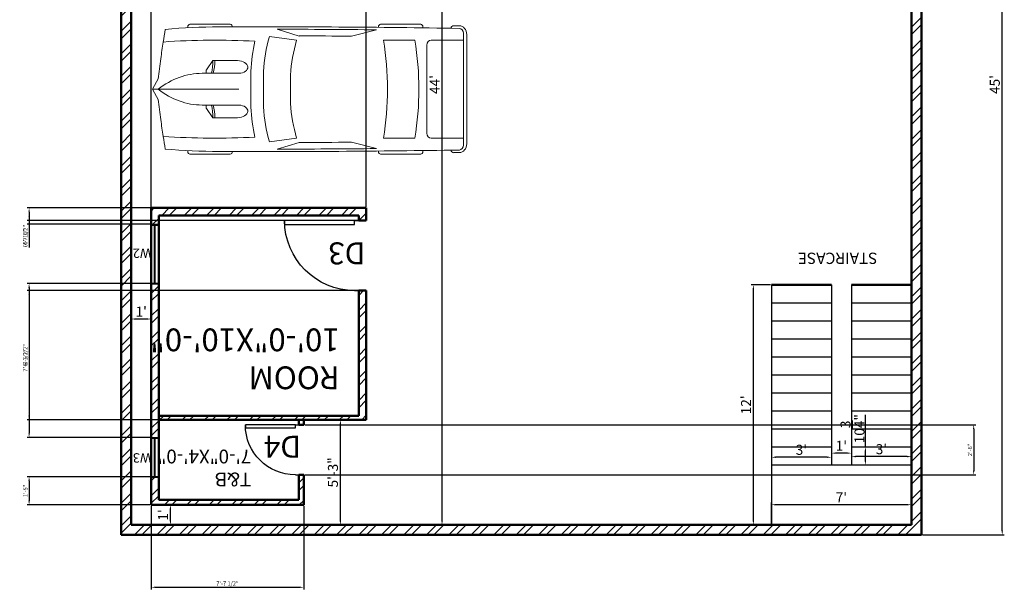
# Model space of a CAD drawing. Units: inches. Extents: x 244 to 2800, y 1060 to 1700.
# Tile 12 of 13: x 2210 to 2800, y 1060 to 1402. Entities that reach past the tile are written whole.
import ezdxf

# ---------------------------------------------------------------- set-up
doc = ezdxf.new("R2010")
doc.units = ezdxf.units.IN
for name, color, linetype, lineweight in [('A-ANNO-DIMS', 2, 'Continuous', 18), ('A-ANNO-TEXT', 1, 'Continuous', 18), ('A-DOOR', 5, 'Continuous', 25), ('A-FLOR-STRS', 6, 'Continuous', 25), ('A-FURN', 9, 'Continuous', 18), ('A-GLAZ', 3, 'Continuous', 25), ('A-WALL', 7, 'Continuous', 50), ('A-WALL-PATT', 8, 'Continuous', 13)]:
    doc.layers.add(name, color=color, linetype=linetype, lineweight=lineweight)
doc.styles.get("Standard").update_dxf_attribs({"font": 'arial.ttf'})
doc.dimstyles.new('ISO-25', dxfattribs={"dimtxt": 2.5, "dimasz": 2.5, "dimexe": 1.25, "dimexo": 0.625, "dimtad": 1, "dimlunit": 4, "dimtxsty": 'Standard', "dimcen": 2.5, "dimadec": 0, "dimazin": 0, "dimtfac": 1, "dimtmove": 0, "dimatfit": 3, "dimfxl": 1, "dimarcsym": 0})

# ---------------------------------------------------------------- blocks, each defined once
blk = doc.blocks.new('*U2')
for p, q in [((0, 0), (0, -5)), ((30, 0), (30, -5))]:
    blk.add_line(p, q)
blk.add_lwpolyline([(0, 0), (0, 30), (1.75, 30), (1.75, 0)], close=True)
blk.add_arc((0, 0), 30, 0, 90)
blk = doc.blocks.new('*D9')
at = {"layer": 'A-ANNO-DIMS', "color": 0, "lineweight": -2, "transparency": 16777216}
for p, q in [((2751.08, 1632.99), (2800.17, 1632.99)), ((2798.92, 1095.49), (2798.92, 1630.49)), ((2751.08, 1092.99), (2800.17, 1092.99))]:
    blk.add_line(p, q, dxfattribs=at)
at = {"layer": 'A-ANNO-DIMS', "color": 0, "transparency": 16777216}
for points in [[(2798.5, 1630.49), (2799.34, 1630.49), (2798.92, 1632.99)], [(2798.5, 1095.49), (2799.34, 1095.49), (2798.92, 1092.99)]]:
    blk.add_solid(points, dxfattribs=at)
at = {"layer": 'Defpoints', "color": 0, "transparency": 16777216}
for p in [(2750.46, 1632.99), (2798.92, 1632.99), (2750.46, 1092.99)]:
    blk.add_point(p, dxfattribs=at)
at = {"layer": 'A-ANNO-DIMS', "color": 0, "transparency": 16777216, "insert": (2795.24, 1362.99), "char_height": 6, "attachment_point": 5, "rotation": 90}
blk.add_mtext("45'", dxfattribs=at)
blk = doc.blocks.new('*D15')
at = {"layer": 'A-ANNO-DIMS', "color": 0, "lineweight": -2, "transparency": 16777216}
for p, q in [((2276.46, 1216.94), (2276.46, 1223.68)), ((2288.46, 1216.94), (2288.46, 1223.68)), ((2285.96, 1222.43), (2278.96, 1222.43))]:
    blk.add_line(p, q, dxfattribs=at)
at = {"layer": 'A-ANNO-DIMS', "color": 0, "transparency": 16777216}
for points in [[(2278.96, 1222.84), (2278.96, 1222.01), (2276.46, 1222.43)], [(2285.96, 1222.84), (2285.96, 1222.01), (2288.46, 1222.43)]]:
    blk.add_solid(points, dxfattribs=at)
at = {"layer": 'Defpoints', "color": 0, "transparency": 16777216}
for p in [(2276.46, 1222.43), (2276.46, 1216.32), (2288.46, 1216.32)]:
    blk.add_point(p, dxfattribs=at)
at = {"layer": 'A-ANNO-DIMS', "color": 0, "transparency": 16777216, "insert": (2282.46, 1226.06), "char_height": 6, "attachment_point": 5}
blk.add_mtext("1'", dxfattribs=at)
blk = doc.blocks.new('*D16')
at = {"layer": 'A-ANNO-DIMS', "color": 0, "lineweight": -2, "transparency": 16777216}
for p, q in [((2305.77, 1110.99), (2298.74, 1110.99)), ((2299.99, 1101.49), (2299.99, 1108.49)), ((2305.77, 1098.99), (2298.74, 1098.99))]:
    blk.add_line(p, q, dxfattribs=at)
at = {"layer": 'A-ANNO-DIMS', "color": 0, "transparency": 16777216}
for points in [[(2299.57, 1108.49), (2300.41, 1108.49), (2299.99, 1110.99)], [(2299.57, 1101.49), (2300.41, 1101.49), (2299.99, 1098.99)]]:
    blk.add_solid(points, dxfattribs=at)
at = {"layer": 'Defpoints', "color": 0, "transparency": 16777216}
for p in [(2299.99, 1110.99), (2306.39, 1110.99), (2306.39, 1098.99)]:
    blk.add_point(p, dxfattribs=at)
at = {"layer": 'A-ANNO-DIMS', "color": 0, "transparency": 16777216, "insert": (2296.35, 1104.99), "char_height": 6, "attachment_point": 5, "rotation": 90}
blk.add_mtext("1'", dxfattribs=at)
blk = doc.blocks.new('*D18')
at = {"layer": 'A-ANNO-DIMS', "color": 0, "lineweight": -2, "transparency": 16777216}
for p, q in [((2660.46, 1099.61), (2660.46, 1112.37)), ((2741.96, 1111.12), (2662.96, 1111.12)), ((2744.46, 1099.61), (2744.46, 1112.37))]:
    blk.add_line(p, q, dxfattribs=at)
at = {"layer": 'A-ANNO-DIMS', "color": 0, "transparency": 16777216}
for points in [[(2662.96, 1111.54), (2662.96, 1110.7), (2660.46, 1111.12)], [(2741.96, 1111.54), (2741.96, 1110.7), (2744.46, 1111.12)]]:
    blk.add_solid(points, dxfattribs=at)
at = {"layer": 'Defpoints', "color": 0, "transparency": 16777216}
for p in [(2660.46, 1111.12), (2660.46, 1098.99), (2744.46, 1098.99)]:
    blk.add_point(p, dxfattribs=at)
at = {"layer": 'A-ANNO-DIMS', "color": 0, "transparency": 16777216, "insert": (2702.46, 1114.74), "char_height": 6, "attachment_point": 5}
blk.add_mtext("7'", dxfattribs=at)
blk = doc.blocks.new('*D19')
at = {"layer": 'A-ANNO-DIMS', "color": 0, "lineweight": -2, "transparency": 16777216}
for p, q in [((2708.46, 1145.16), (2708.46, 1138.69)), ((2741.96, 1139.94), (2710.96, 1139.94)), ((2744.46, 1145.16), (2744.46, 1138.69))]:
    blk.add_line(p, q, dxfattribs=at)
at = {"layer": 'A-ANNO-DIMS', "color": 0, "transparency": 16777216}
for points in [[(2710.96, 1140.36), (2710.96, 1139.52), (2708.46, 1139.94)], [(2741.96, 1140.36), (2741.96, 1139.52), (2744.46, 1139.94)]]:
    blk.add_solid(points, dxfattribs=at)
at = {"layer": 'Defpoints', "color": 0, "transparency": 16777216}
for p in [(2708.46, 1145.79), (2744.46, 1145.79), (2708.46, 1139.94)]:
    blk.add_point(p, dxfattribs=at)
at = {"layer": 'A-ANNO-DIMS', "color": 0, "transparency": 16777216, "insert": (2726.46, 1143.63), "char_height": 6, "attachment_point": 5}
blk.add_mtext("3'", dxfattribs=at)
blk = doc.blocks.new('*D20')
at = {"layer": 'A-ANNO-DIMS', "color": 0, "lineweight": -2, "transparency": 16777216}
for p, q in [((2716.85, 1145.79), (2716.85, 1165.08)), ((2709.08, 1145.79), (2718.1, 1145.79)), ((2716.85, 1137.49), (2716.85, 1143.29)), ((2709.08, 1134.99), (2718.1, 1134.99))]:
    blk.add_line(p, q, dxfattribs=at)
at = {"layer": 'A-ANNO-DIMS', "color": 0, "transparency": 16777216}
for points in [[(2716.43, 1143.29), (2717.27, 1143.29), (2716.85, 1145.79)], [(2716.43, 1137.49), (2717.27, 1137.49), (2716.85, 1134.99)]]:
    blk.add_solid(points, dxfattribs=at)
at = {"layer": 'Defpoints', "color": 0, "transparency": 16777216}
for p in [(2708.46, 1145.79), (2716.85, 1145.79), (2708.46, 1134.99)]:
    blk.add_point(p, dxfattribs=at)
at = {"layer": 'A-ANNO-DIMS', "color": 0, "transparency": 16777216, "insert": (2709.11, 1156.68), "char_height": 6, "attachment_point": 5, "rotation": 90}
blk.add_mtext('10{\\H1x;\\S3/4;}"', dxfattribs=at)
blk = doc.blocks.new('*D21')
at = {"layer": 'A-ANNO-DIMS', "color": 0, "lineweight": -2, "transparency": 16777216}
for p, q in [((2696.46, 1145.16), (2696.46, 1140.78)), ((2705.96, 1142.03), (2698.96, 1142.03)), ((2708.46, 1145.16), (2708.46, 1140.78))]:
    blk.add_line(p, q, dxfattribs=at)
at = {"layer": 'A-ANNO-DIMS', "color": 0, "transparency": 16777216}
for points in [[(2698.96, 1142.45), (2698.96, 1141.62), (2696.46, 1142.03)], [(2705.96, 1142.45), (2705.96, 1141.62), (2708.46, 1142.03)]]:
    blk.add_solid(points, dxfattribs=at)
at = {"layer": 'Defpoints', "color": 0, "transparency": 16777216}
for p in [(2696.46, 1145.79), (2708.46, 1145.79), (2696.46, 1142.03)]:
    blk.add_point(p, dxfattribs=at)
at = {"layer": 'A-ANNO-DIMS', "color": 0, "transparency": 16777216, "insert": (2702.46, 1145.67), "char_height": 6, "attachment_point": 5}
blk.add_mtext("1'", dxfattribs=at)
blk = doc.blocks.new('*D22')
at = {"layer": 'A-ANNO-DIMS', "color": 0, "lineweight": -2, "transparency": 16777216}
for p, q in [((2660.46, 1143.51), (2660.46, 1138.32)), ((2696.46, 1143.51), (2696.46, 1138.32)), ((2693.96, 1139.57), (2662.96, 1139.57))]:
    blk.add_line(p, q, dxfattribs=at)
at = {"layer": 'A-ANNO-DIMS', "color": 0, "transparency": 16777216}
for points in [[(2662.96, 1139.99), (2662.96, 1139.16), (2660.46, 1139.57)], [(2693.96, 1139.99), (2693.96, 1139.16), (2696.46, 1139.57)]]:
    blk.add_solid(points, dxfattribs=at)
at = {"layer": 'Defpoints', "color": 0, "transparency": 16777216}
for p in [(2660.46, 1144.13), (2696.46, 1144.13), (2660.46, 1139.57)]:
    blk.add_point(p, dxfattribs=at)
at = {"layer": 'A-ANNO-DIMS', "color": 0, "transparency": 16777216, "insert": (2678.46, 1143.26), "char_height": 6, "attachment_point": 5}
blk.add_mtext("3'", dxfattribs=at)
blk = doc.blocks.new('*D23')
at = {"layer": 'A-ANNO-DIMS', "color": 0, "lineweight": -2, "transparency": 16777216}
for p, q in [((2659.83, 1242.99), (2648.4, 1242.99)), ((2649.65, 1101.49), (2649.65, 1240.49)), ((2659.83, 1098.99), (2648.4, 1098.99))]:
    blk.add_line(p, q, dxfattribs=at)
at = {"layer": 'A-ANNO-DIMS', "color": 0, "transparency": 16777216}
for points in [[(2649.24, 1240.49), (2650.07, 1240.49), (2649.65, 1242.99)], [(2649.24, 1101.49), (2650.07, 1101.49), (2649.65, 1098.99)]]:
    blk.add_solid(points, dxfattribs=at)
at = {"layer": 'Defpoints', "color": 0, "transparency": 16777216}
for p in [(2649.65, 1242.99), (2660.46, 1242.99), (2660.46, 1098.99)]:
    blk.add_point(p, dxfattribs=at)
at = {"layer": 'A-ANNO-DIMS', "color": 0, "transparency": 16777216, "insert": (2646.02, 1170.99), "char_height": 6, "attachment_point": 5, "rotation": 90}
blk.add_mtext("12'", dxfattribs=at)
blk = doc.blocks.new('*D24')
at = {"layer": 'A-ANNO-DIMS', "color": 0, "lineweight": -2, "transparency": 16777216}
for p, q in [((2407.43, 1161.99), (2400.69, 1161.99)), ((2401.94, 1101.49), (2401.94, 1159.49)), ((2407.43, 1098.99), (2400.69, 1098.99))]:
    blk.add_line(p, q, dxfattribs=at)
at = {"layer": 'A-ANNO-DIMS', "color": 0, "transparency": 16777216}
for points in [[(2401.52, 1159.49), (2402.36, 1159.49), (2401.94, 1161.99)], [(2401.52, 1101.49), (2402.36, 1101.49), (2401.94, 1098.99)]]:
    blk.add_solid(points, dxfattribs=at)
at = {"layer": 'Defpoints', "color": 0, "transparency": 16777216}
for p in [(2401.94, 1161.99), (2408.06, 1161.99), (2408.06, 1098.99)]:
    blk.add_point(p, dxfattribs=at)
at = {"layer": 'A-ANNO-DIMS', "color": 0, "transparency": 16777216, "insert": (2398.25, 1130.49), "char_height": 6, "attachment_point": 5, "rotation": 90}
blk.add_mtext('5\'-3"', dxfattribs=at)
blk = doc.blocks.new('*D45')
at = {"layer": 'A-ANNO-DIMS', "color": 0, "lineweight": -2, "transparency": 16777216}
for p, q in [((2478.2, 1626.99), (2461.68, 1626.99)), ((2462.93, 1101.49), (2462.93, 1624.49)), ((2478.2, 1098.99), (2461.68, 1098.99))]:
    blk.add_line(p, q, dxfattribs=at)
at = {"layer": 'A-ANNO-DIMS', "color": 0, "transparency": 16777216}
for points in [[(2462.51, 1624.49), (2463.34, 1624.49), (2462.93, 1626.99)], [(2462.51, 1101.49), (2463.34, 1101.49), (2462.93, 1098.99)]]:
    blk.add_solid(points, dxfattribs=at)
at = {"layer": 'Defpoints', "color": 0, "transparency": 16777216}
for p in [(2462.93, 1626.99), (2478.82, 1626.99), (2478.82, 1098.99)]:
    blk.add_point(p, dxfattribs=at)
at = {"layer": 'A-ANNO-DIMS', "color": 0, "transparency": 16777216, "insert": (2459.3, 1362.99), "char_height": 6, "attachment_point": 5, "rotation": 90}
blk.add_mtext("44'", dxfattribs=at)
blk = doc.blocks.new('*U47')
for p, q in [((21.1, 37.41), (21.1, 36.83)), ((46.55, 38.89), (22.35, 38.89)), ((47.8, 37.39), (47.8, 37.41)), ((87.99, 31.87), (74.76, 35.92)), ((134.31, 35.6), (119.29, 31.78)), ((135.45, 37.07), (135.45, 37.41)), ((136.7, 38.89), (160.9, 38.89)), ((162.15, 37.41), (162.15, 36.77)), ((70.03, 31.54), (86.41, 29.35)), ((186.47, -33.5), (186.47, 33.5)), ((188.4, -32.76), (188.4, 32.76)), ((138.42, 29.35), (157.25, 29.35)), ((164.52, 26.39), (164.52, -26.39)), ((186.47, 29.35), (167.01, 29.35)), ((32.27, 11.63), (36.13, 17.17)), ((36.13, 17.17), (50.94, 17.17)), ((3.27, 6.13), (0.1, 0.41)), ((29.77, 9.51), (51.68, 9.51)), ((32.12, 9.51), (32.12, 11.15)), ((58.92, -10.77), (58.92, 10.77)), ((66.55, -10.53), (66.55, 10.53)), ((82.74, 8.5), (82.74, -8.5)), ((186.47, -10.53), (186.47, 10.53)), ((0, 0), (51.68, 0)), ((0.1, -0.41), (3.27, -6.13)), ((29.77, -9.51), (51.68, -9.51)), ((32.12, -9.51), (32.12, -11.15)), ((32.27, -11.63), (36.13, -17.17)), ((36.13, -17.17), (50.94, -17.17)), ((86.41, -29.35), (70.03, -31.54)), ((157.25, -29.35), (138.42, -29.35)), ((167.01, -29.35), (186.47, -29.35)), ((87.99, -31.87), (74.76, -35.92)), ((134.31, -35.6), (119.29, -31.78)), ((21.1, -37.41), (21.1, -36.83)), ((46.55, -38.89), (22.35, -38.89)), ((47.8, -37.39), (47.8, -37.41)), ((135.45, -37.07), (135.45, -37.41)), ((136.7, -38.89), (160.9, -38.89)), ((162.15, -37.41), (162.15, -36.77))]:
    blk.add_line(p, q)
for centre, major_axis, ratio, start_param, end_param in [((266.03, -27.52), (0, 313.31), 0.842304, 1.367076, 1.39176), ((41.19, -490.86), (0, 528.23), 0.842304, 0.00281, 0.075598), ((22.35, 37.41), (0, -1.48), 0.842304, 3.141593, 4.712389), ((64.48, -10555.62), (0, 10593.03), 0.842304, -0.013397, 0.002797), ((46.55, 37.41), (0, 1.48), 0.842304, -1.570796, 0), ((64.48, -10555.62), (0, -10591.55), 0.842304, 3.133765, 3.140441), ((136.7, 37.41), (0, -1.48), 0.842304, 3.141593, 4.712389), ((160.9, 37.41), (0, 1.48), 0.842304, -1.570796, 0), ((180.63, 35.84), (0, 2.22), 0.842304, -0.013017, 1.249894), ((64.48, -10556.36), (0, 10595.31), 0.842304, -0.013397, -0.013017), ((183.98, 33.5), (0, -2.96), 0.842304, 1.570796, 3.128196), ((183.98, 32.76), (0, -5.25), 0.842304, 1.570796, 3.128196), ((37.47, -593.96), (0, -623.33), 0.842304, 3.096046, 3.200911), ((135.29, 5.39), (0, 81.77), 0.842304, 1.245306, 1.50788), ((95.79, -3666.35), (0, -3698.24), 0.842304, 3.134049, 3.144098), ((259.18, -27.52), (0, -305.3), 0.842304, 4.528606, 4.561838), ((134.4, 5.39), (0, -89.78), 0.842304, 4.449482, 4.652344), ((149.6, 2.8), (0, -79.58), 0.842304, 4.372215, 4.640744), ((17.08, 0), (0, 147.02), 0.842304, 4.511394, 4.913384), ((35.91, 0), (0, 147.02), 0.842304, 4.511394, 4.913384), ((167.01, 26.39), (0, 2.96), 0.842304, 0, 1.570796), ((-204.49, 52.4), (0, -250.96), 0.842304, 1.385369, 1.434372), ((13.04, 17.01), (0, 27.42), 0.842304, 4.435146, 4.718221), ((14.2, 17.01), (0, 27.42), 0.842304, 4.435146, 4.718221), ((50.79, 13.34), (6.34, -0.36), 0.603834, -1.395552, 1.581315), ((29.77, -46.66), (0, 56.17), 0.842304, 0, 0.590319), ((32.75, 11.15), (0, 0.74), 0.842304, 0.879714, 1.570796), ((0.62, 0), (0, -0.74), 0.842304, 4.131459, 5.293319), ((29.77, 46.66), (0, 56.17), 0.842304, 2.551274, 3.141593), ((-204.49, -52.4), (0, 250.96), 0.842304, -1.434372, -1.385369), ((32.75, -11.15), (0, -0.74), 0.842304, 4.712389, 5.403472), ((13.04, -17.01), (0, -27.42), 0.842304, 1.564964, 1.848039), ((14.2, -17.01), (0, -27.42), 0.842304, 1.564964, 1.848039), ((134.4, -5.39), (0, -89.78), 0.842304, -1.510751, -1.307889), ((135.29, -5.39), (0, -81.77), 0.842304, -1.50788, -1.245306), ((149.6, -2.8), (0, -79.58), 0.842304, -1.499151, -1.230623), ((259.18, 27.52), (0, 305.3), 0.842304, 1.721348, 1.754579), ((266.03, 27.52), (0, 313.31), 0.842304, 1.749832, 1.774517), ((37.47, 593.96), (0, -623.33), 0.842304, -0.059319, 0.045547), ((167.01, -26.39), (0, -2.96), 0.842304, 4.712389, 6.283185), ((95.79, 3666.35), (0, -3698.24), 0.842304, -0.002505, 0.007544), ((183.98, -33.5), (0, 2.96), 0.842304, 3.15499, 4.712389), ((183.98, -32.76), (0, -5.25), 0.842304, 0.013397, 1.570796), ((41.19, 490.86), (0, -528.23), 0.842304, -0.075598, -0.00281), ((22.35, -37.41), (0, 1.48), 0.842304, 1.570796, 3.141593), ((64.48, 10555.62), (0, 10593.03), 0.842304, 3.138796, 3.15499), ((46.55, -37.41), (0, -1.48), 0.842304, 0, 1.570796), ((64.48, 10555.62), (0, -10591.55), 0.842304, 0.001152, 0.007828), ((136.7, -37.41), (0, -1.48), 0.842304, -1.570796, 0), ((160.9, -37.41), (0, 1.48), 0.842304, 3.141593, 4.712389), ((180.63, -35.84), (0, -2.22), 0.842304, -1.249894, 0.013017), ((64.48, 10556.36), (0, 10595.31), 0.842304, 3.15461, 3.15499)]:
    blk.add_ellipse(centre, major_axis=major_axis, ratio=ratio, start_param=start_param, end_param=end_param)
at = {"extrusion": (0, 0, -1)}
blk.add_ellipse((50.79, -13.34), major_axis=(6.34, 0.36), ratio=0.603834, start_param=-1.395552, end_param=1.581315, dxfattribs=at)
blk = doc.blocks.new('*D148')
at = {"layer": 'A-ANNO-DIMS', "color": 0, "lineweight": -2, "transparency": 16777216}
for p, q in [((2288.46, 1289.61), (2288.46, 1665.59)), ((2417.46, 1289.61), (2417.46, 1665.59)), ((2290.96, 1664.34), (2414.96, 1664.34))]:
    blk.add_line(p, q, dxfattribs=at)
at = {"layer": 'A-ANNO-DIMS', "color": 0, "transparency": 16777216}
for points in [[(2290.96, 1664.75), (2290.96, 1663.92), (2288.46, 1664.34)], [(2414.96, 1664.75), (2414.96, 1663.92), (2417.46, 1664.34)]]:
    blk.add_solid(points, dxfattribs=at)
at = {"layer": 'Defpoints', "color": 0, "transparency": 16777216}
for p in [(2417.46, 1664.34), (2288.46, 1288.99), (2417.46, 1288.99)]:
    blk.add_point(p, dxfattribs=at)
at = {"layer": 'A-ANNO-DIMS', "color": 0, "transparency": 16777216, "insert": (2352.96, 1666.24), "char_height": 2.5, "attachment_point": 5}
blk.add_mtext('10\'-9"', dxfattribs=at)
blk = doc.blocks.new('*D149')
at = {"layer": 'A-ANNO-DIMS', "color": 0, "lineweight": -2, "transparency": 16777216}
for p, q in [((2287.83, 1288.99), (2213.97, 1288.99)), ((2215.22, 1286.49), (2215.22, 1281.7)), ((2287.83, 1279.2), (2213.97, 1279.2)), ((2215.22, 1279.2), (2215.22, 1266.86))]:
    blk.add_line(p, q, dxfattribs=at)
at = {"layer": 'A-ANNO-DIMS', "color": 0, "transparency": 16777216}
for points in [[(2214.81, 1286.49), (2215.64, 1286.49), (2215.22, 1288.99)], [(2214.81, 1281.7), (2215.64, 1281.7), (2215.22, 1279.2)]]:
    blk.add_solid(points, dxfattribs=at)
at = {"layer": 'Defpoints', "color": 0, "transparency": 16777216}
for p in [(2288.46, 1288.99), (2215.22, 1279.2), (2288.46, 1279.2)]:
    blk.add_point(p, dxfattribs=at)
at = {"layer": 'A-ANNO-DIMS', "color": 0, "transparency": 16777216, "insert": (2213.32, 1271.78), "char_height": 2.5, "attachment_point": 5, "rotation": 90}
blk.add_mtext('0\'-10"', dxfattribs=at)
blk = doc.blocks.new('*D150')
at = {"layer": 'A-ANNO-DIMS', "color": 0, "lineweight": -2, "transparency": 16777216}
for p, q in [((2287.83, 1243.73), (2213.97, 1243.73)), ((2215.22, 1241.23), (2215.22, 1153.92)), ((2287.83, 1151.42), (2213.97, 1151.42))]:
    blk.add_line(p, q, dxfattribs=at)
at = {"layer": 'A-ANNO-DIMS', "color": 0, "transparency": 16777216}
for points in [[(2214.81, 1241.23), (2215.64, 1241.23), (2215.22, 1243.73)], [(2214.81, 1153.92), (2215.64, 1153.92), (2215.22, 1151.42)]]:
    blk.add_solid(points, dxfattribs=at)
at = {"layer": 'Defpoints', "color": 0, "transparency": 16777216}
for p in [(2288.46, 1243.73), (2215.22, 1151.42), (2288.46, 1151.42)]:
    blk.add_point(p, dxfattribs=at)
at = {"layer": 'A-ANNO-DIMS', "color": 0, "transparency": 16777216, "insert": (2213.31, 1197.57), "char_height": 2.5, "attachment_point": 5, "rotation": 90}
blk.add_mtext('7\'-8 1/2"', dxfattribs=at)
blk = doc.blocks.new('*D151')
at = {"layer": 'A-ANNO-DIMS', "color": 0, "lineweight": -2, "transparency": 16777216}
for p, q in [((2287.83, 1127.9), (2213.97, 1127.9)), ((2215.22, 1125.4), (2215.22, 1113.49)), ((2287.83, 1110.99), (2213.97, 1110.99))]:
    blk.add_line(p, q, dxfattribs=at)
at = {"layer": 'A-ANNO-DIMS', "color": 0, "transparency": 16777216}
for points in [[(2214.81, 1125.4), (2215.64, 1125.4), (2215.22, 1127.9)], [(2214.81, 1113.49), (2215.64, 1113.49), (2215.22, 1110.99)]]:
    blk.add_solid(points, dxfattribs=at)
at = {"layer": 'Defpoints', "color": 0, "transparency": 16777216}
for p in [(2288.46, 1127.9), (2215.22, 1110.99), (2288.46, 1110.99)]:
    blk.add_point(p, dxfattribs=at)
at = {"layer": 'A-ANNO-DIMS', "color": 0, "transparency": 16777216, "insert": (2213.32, 1119.44), "char_height": 2.5, "attachment_point": 5, "rotation": 90}
blk.add_mtext('1\'-5"', dxfattribs=at)
blk = doc.blocks.new('*D152')
at = {"layer": 'A-ANNO-DIMS', "color": 0, "lineweight": -2, "transparency": 16777216}
for p, q in [((2416.83, 1288.99), (2213.97, 1288.99)), ((2215.22, 1286.49), (2215.22, 1283.99)), ((2416.83, 1281.49), (2213.97, 1281.49)), ((2215.22, 1281.49), (2215.22, 1265.27))]:
    blk.add_line(p, q, dxfattribs=at)
at = {"layer": 'A-ANNO-DIMS', "color": 0, "transparency": 16777216}
for points in [[(2214.81, 1286.49), (2215.64, 1286.49), (2215.22, 1288.99)], [(2214.81, 1283.99), (2215.64, 1283.99), (2215.22, 1281.49)]]:
    blk.add_solid(points, dxfattribs=at)
at = {"layer": 'Defpoints', "color": 0, "transparency": 16777216}
for p in [(2417.46, 1288.99), (2215.22, 1281.49), (2417.46, 1281.49)]:
    blk.add_point(p, dxfattribs=at)
at = {"layer": 'A-ANNO-DIMS', "color": 0, "transparency": 16777216, "insert": (2213.31, 1272.13), "char_height": 2.5, "attachment_point": 5, "rotation": 90}
blk.add_mtext('0\'-7 1/2"', dxfattribs=at)
blk = doc.blocks.new('*D153')
at = {"layer": 'A-ANNO-DIMS', "color": 0, "lineweight": -2, "transparency": 16777216}
for p, q in [((2416.83, 1239.49), (2213.97, 1239.49)), ((2215.22, 1236.99), (2215.22, 1164.49)), ((2416.83, 1161.99), (2213.97, 1161.99))]:
    blk.add_line(p, q, dxfattribs=at)
at = {"layer": 'A-ANNO-DIMS', "color": 0, "transparency": 16777216}
for points in [[(2214.81, 1236.99), (2215.64, 1236.99), (2215.22, 1239.49)], [(2214.81, 1164.49), (2215.64, 1164.49), (2215.22, 1161.99)]]:
    blk.add_solid(points, dxfattribs=at)
at = {"layer": 'Defpoints', "color": 0, "transparency": 16777216}
for p in [(2417.46, 1239.49), (2215.22, 1161.99), (2417.46, 1161.99)]:
    blk.add_point(p, dxfattribs=at)
at = {"layer": 'A-ANNO-DIMS', "color": 0, "transparency": 16777216, "insert": (2213.31, 1200.74), "char_height": 2.5, "attachment_point": 5, "rotation": 90}
blk.add_mtext('6\'-5 1/2"', dxfattribs=at)
blk = doc.blocks.new('*D154')
at = {"layer": 'A-ANNO-DIMS', "color": 0, "lineweight": -2, "transparency": 16777216}
for p, q in [((2380.58, 1158.99), (2783.06, 1158.99)), ((2781.81, 1156.49), (2781.81, 1131.49)), ((2380.58, 1128.99), (2783.06, 1128.99))]:
    blk.add_line(p, q, dxfattribs=at)
at = {"layer": 'A-ANNO-DIMS', "color": 0, "transparency": 16777216}
for points in [[(2781.39, 1156.49), (2782.22, 1156.49), (2781.81, 1158.99)], [(2781.39, 1131.49), (2782.22, 1131.49), (2781.81, 1128.99)]]:
    blk.add_solid(points, dxfattribs=at)
at = {"layer": 'Defpoints', "color": 0, "transparency": 16777216}
for p in [(2379.96, 1158.99), (2379.96, 1128.99), (2781.81, 1128.99)]:
    blk.add_point(p, dxfattribs=at)
at = {"layer": 'A-ANNO-DIMS', "color": 0, "transparency": 16777216, "insert": (2779.91, 1143.99), "char_height": 2.5, "attachment_point": 5, "rotation": 90}
blk.add_mtext('2\'-6"', dxfattribs=at)
blk = doc.blocks.new('*D155')
at = {"layer": 'A-ANNO-DIMS', "color": 0, "lineweight": -2, "transparency": 16777216}
for p, q in [((2288.46, 1110.36), (2288.46, 1060.39)), ((2379.96, 1110.36), (2379.96, 1060.39)), ((2290.96, 1061.64), (2377.46, 1061.64))]:
    blk.add_line(p, q, dxfattribs=at)
at = {"layer": 'A-ANNO-DIMS', "color": 0, "transparency": 16777216}
for points in [[(2290.96, 1062.05), (2290.96, 1061.22), (2288.46, 1061.64)], [(2377.46, 1062.05), (2377.46, 1061.22), (2379.96, 1061.64)]]:
    blk.add_solid(points, dxfattribs=at)
at = {"layer": 'Defpoints', "color": 0, "transparency": 16777216}
for p in [(2288.46, 1110.99), (2379.96, 1110.99), (2379.96, 1061.64)]:
    blk.add_point(p, dxfattribs=at)
at = {"layer": 'A-ANNO-DIMS', "color": 0, "transparency": 16777216, "insert": (2334.21, 1063.55), "char_height": 2.5, "attachment_point": 5}
blk.add_mtext('7\'-7 1/2"', dxfattribs=at)

msp = doc.modelspace()

# ---------------------------------------------------------------- hatches: boundary and pattern name
at = {"layer": 'A-WALL-PATT'}
h = msp.add_hatch(dxfattribs=at)
h.set_pattern_fill('ANSI32', color=256)
h.paths.add_polyline_path([(2750.457, 1632.986), (2270.457, 1632.986), (2270.457, 1092.986), (2750.457, 1092.986)])
h.paths.add_polyline_path([(2276.457, 1626.986), (2744.457, 1626.986), (2744.457, 1098.986), (2660.457, 1098.986), (2276.457, 1098.986)], flags=16)
h.paths.add_polyline_path([(2288.457, 1288.986), (2417.457, 1288.986), (2417.457, 1281.486), (2412.957, 1281.486), (2412.957, 1284.486), (2292.957, 1284.486), (2292.957, 1164.486), (2412.957, 1164.486), (2412.957, 1239.486), (2417.457, 1239.486), (2417.457, 1161.986), (2379.957, 1161.986), (2379.957, 1158.986), (2376.957, 1158.986), (2376.957, 1161.986), (2292.957, 1161.986), (2292.957, 1113.986), (2376.957, 1113.986), (2376.957, 1128.986), (2379.957, 1128.986), (2379.957, 1110.986), (2288.457, 1110.986)], flags=0)
h.paths.add_polyline_path([(2288.457, 1279.202), (2292.957, 1279.202), (2292.957, 1243.232), (2288.457, 1243.232)], flags=0)
h.paths.add_polyline_path([(2290.907, 1278.702), (2290.907, 1243.732), (2290.507, 1243.732), (2290.507, 1278.702)], flags=0)
h.paths.add_polyline_path([(2288.457, 1151.417), (2292.957, 1151.417), (2292.957, 1127.404), (2288.457, 1127.404)], flags=0)
h.paths.add_polyline_path([(2290.907, 1150.917), (2290.907, 1127.904), (2290.507, 1127.904), (2290.507, 1150.917)], flags=0)
h.paths.add_polyline_path([(2279.972, 1551.986), (2279.972, 1623.986), (2363.972, 1623.986), (2363.972, 1551.986)], flags=0)
h.paths.add_polyline_path([(2660.457, 1242.986), (2696.457, 1242.986), (2696.457, 1134.986), (2708.457, 1134.986), (2708.457, 1242.986), (2744.457, 1242.986), (2744.457, 1134.986), (2660.457, 1134.986)], flags=0)
h.paths.add_polyline_path([(2379.957, 1128.986), (2376.957, 1128.986), (2376.957, 1113.986), (2292.957, 1113.986), (2292.957, 1127.404), (2288.457, 1127.404), (2288.457, 1110.986), (2379.957, 1110.986)], flags=0)
h.paths.add_polyline_path([(2417.457, 1239.486), (2412.957, 1239.486), (2412.957, 1164.486), (2292.957, 1164.486), (2292.957, 1161.986), (2376.957, 1161.986), (2417.457, 1161.986)], flags=0)
h.paths.add_polyline_path([(2289.96, 1267.789), (2275.356, 1267.789), (2275.356, 1256.194), (2289.96, 1256.194)], flags=24)
h.paths.add_polyline_path([(2289.96, 1145.072), (2275.356, 1145.072), (2275.356, 1133.477), (2289.96, 1133.477)], flags=24)
h.paths.add_polyline_path([(2406.937, 1224.517), (2290.255, 1224.517), (2290.255, 1173.588), (2406.937, 1173.588)], flags=8)
h.paths.add_polyline_path([(2351.026, 1148.815), (2293.304, 1148.815), (2293.304, 1118.024), (2351.026, 1118.024)], flags=8)
h.paths.add_polyline_path([(2383.007, 1159.633), (2352.857, 1159.633), (2352.857, 1132.452), (2383.007, 1132.452)], flags=8)
h.paths.add_polyline_path([(2421.657, 1275.631), (2391.507, 1275.631), (2391.507, 1248.45), (2421.657, 1248.45)], flags=8)
h.paths.add_polyline_path([(2394.334, 1573.477), (2394.334, 1615.869), (2371.88, 1615.869), (2371.88, 1573.477)], flags=8)
h.paths.add_polyline_path([(2726.202, 1266.003), (2669.205, 1266.003), (2669.205, 1252.05), (2726.202, 1252.05)], flags=8)
h = msp.add_hatch(dxfattribs=at)
h.set_pattern_fill('ANSI32', color=256)
h.paths.add_polyline_path([(2417.457, 1288.986), (2288.457, 1288.986), (2288.457, 1279.202), (2292.957, 1279.202), (2292.957, 1284.486), (2412.957, 1284.486), (2412.957, 1281.486), (2417.457, 1281.486)])
h = msp.add_hatch(dxfattribs=at)
h.set_pattern_fill('ANSI32', color=256)
h.paths.add_polyline_path([(2292.957, 1243.232), (2288.457, 1243.232), (2288.457, 1151.417), (2292.957, 1151.417)])
h = msp.add_hatch(dxfattribs=at)
h.set_pattern_fill('ANSI32', color=256)
h.paths.add_polyline_path([(2417.457, 1239.486), (2412.957, 1239.486), (2412.957, 1164.486), (2292.957, 1164.486), (2292.957, 1161.986), (2417.457, 1161.986)])
h = msp.add_hatch(dxfattribs=at)
h.set_pattern_fill('ANSI32', color=256)
h.paths.add_polyline_path([(2379.957, 1110.986), (2379.957, 1128.986), (2376.957, 1128.986), (2376.957, 1113.986), (2292.957, 1113.986), (2292.957, 1127.404), (2288.457, 1127.404), (2288.457, 1110.986)])

# ---------------------------------------------------------------- linework, layer by layer
at = {"layer": 'A-FLOR-STRS'}
for p, q in [((2660.457, 1242.986), (2696.457, 1242.986)), ((2660.457, 1242.986), (2660.457, 1098.986)), ((2660.457, 1242.986), (2696.457, 1242.986)), ((2696.457, 1242.986), (2696.457, 1134.986)), ((2708.457, 1242.986), (2708.457, 1134.986)), ((2708.457, 1242.986), (2744.457, 1242.986)), ((2708.457, 1242.986), (2744.457, 1242.986)), ((2744.457, 1242.986), (2744.457, 1098.986)), ((2660.457, 1232.186), (2696.457, 1232.186)), ((2708.457, 1232.186), (2744.457, 1232.186)), ((2660.457, 1221.386), (2696.457, 1221.386)), ((2708.457, 1221.386), (2744.457, 1221.386)), ((2660.457, 1210.586), (2696.457, 1210.586)), ((2708.457, 1210.586), (2744.457, 1210.586)), ((2660.457, 1199.786), (2696.457, 1199.786)), ((2708.457, 1199.786), (2744.457, 1199.786)), ((2660.457, 1188.986), (2696.457, 1188.986)), ((2708.457, 1188.986), (2744.457, 1188.986)), ((2660.457, 1178.186), (2696.457, 1178.186)), ((2708.457, 1178.186), (2744.457, 1178.186)), ((2660.457, 1167.386), (2696.457, 1167.386)), ((2708.457, 1167.386), (2744.457, 1167.386)), ((2660.457, 1156.586), (2696.457, 1156.586)), ((2708.457, 1156.586), (2744.457, 1156.586)), ((2660.457, 1145.786), (2696.457, 1145.786)), ((2708.457, 1145.786), (2744.457, 1145.786)), ((2660.457, 1134.986), (2744.457, 1134.986)), ((2660.457, 1098.986), (2744.457, 1098.986))]:
    msp.add_line(p, q, dxfattribs=at)
at = {"layer": 'A-GLAZ'}
for p, q in [((2288.457, 1243.232), (2288.457, 1279.202)), ((2288.457, 1279.202), (2292.957, 1279.202)), ((2288.457, 1278.702), (2292.957, 1278.702)), ((2290.507, 1243.732), (2290.507, 1278.702)), ((2290.907, 1243.732), (2290.907, 1278.702)), ((2292.957, 1279.202), (2292.957, 1243.232)), ((2292.957, 1243.732), (2288.457, 1243.732)), ((2292.957, 1243.232), (2288.457, 1243.232)), ((2288.457, 1127.404), (2288.457, 1151.417)), ((2288.457, 1151.417), (2292.957, 1151.417)), ((2288.457, 1150.917), (2292.957, 1150.917)), ((2290.507, 1127.904), (2290.507, 1150.917)), ((2290.907, 1127.904), (2290.907, 1150.917)), ((2292.957, 1151.417), (2292.957, 1127.404)), ((2292.957, 1127.904), (2288.457, 1127.904)), ((2292.957, 1127.404), (2288.457, 1127.404))]:
    msp.add_line(p, q, dxfattribs=at)
at = {"layer": 'A-WALL'}
for p, q in [((2270.457, 1632.986), (2270.457, 1092.986)), ((2750.457, 1092.986), (2750.457, 1632.986)), ((2276.457, 1626.986), (2276.457, 1098.986)), ((2744.457, 1098.986), (2744.457, 1626.986)), ((2288.457, 1288.986), (2417.457, 1288.986)), ((2288.457, 1288.986), (2288.457, 1110.986)), ((2417.457, 1288.986), (2417.457, 1281.486)), ((2292.957, 1284.486), (2412.957, 1284.486)), ((2292.957, 1284.486), (2292.957, 1113.986)), ((2412.957, 1284.486), (2412.957, 1281.486)), ((2412.957, 1284.486), (2412.957, 1281.486)), ((2412.957, 1281.486), (2417.457, 1281.486)), ((2660.457, 1242.986), (2696.457, 1242.986)), ((2708.457, 1242.986), (2744.457, 1242.986)), ((2417.457, 1239.486), (2412.957, 1239.486)), ((2412.957, 1239.486), (2412.957, 1164.486)), ((2417.457, 1239.486), (2417.457, 1161.986)), ((2412.957, 1164.486), (2292.957, 1164.486)), ((2417.457, 1161.986), (2292.957, 1161.986)), ((2376.957, 1161.986), (2376.957, 1158.986)), ((2376.957, 1161.986), (2376.957, 1158.986)), ((2376.957, 1158.986), (2379.957, 1158.986)), ((2379.957, 1161.986), (2379.957, 1158.986)), ((2379.957, 1128.986), (2376.957, 1128.986)), ((2376.957, 1128.986), (2376.957, 1113.986)), ((2379.957, 1128.986), (2379.957, 1110.986)), ((2288.457, 1110.986), (2379.957, 1110.986)), ((2292.957, 1113.986), (2376.957, 1113.986)), ((2276.457, 1098.986), (2744.457, 1098.986)), ((2270.457, 1092.986), (2750.457, 1092.986))]:
    msp.add_line(p, q, dxfattribs=at)

# ---------------------------------------------------------------- block references
at = {"layer": 'A-DOOR', "xscale": -1.399999999999999, "yscale": 1.399999999999999, "zscale": 1.399999999999999, "rotation": 90}
msp.add_blockref('*U2', (2410.457, 1281.486), dxfattribs=at)
at = {"layer": 'A-DOOR', "xscale": -1, "rotation": 90}
msp.add_blockref('*U2', (2374.957, 1158.986), dxfattribs=at)
at = {"layer": 'A-FURN'}
msp.add_blockref('*U47', (2289.297, 1360.191), dxfattribs=at)

# ---------------------------------------------------------------- texts
at = {"layer": 'A-ANNO-TEXT', "attachment_point": 1, "rotation": 180}
for s, width, gutter_width, insert, char_height in [('W2', 2.91536, 28.132, (2288.457, 1259.067), 5.6265), ('D3', 20.58737, 65.951, (2416.938, 1255.185), 13.1902), ('STAIRCASE', 2.71935, 33.854, (2724.085, 1255.419), 6.7708), ('ROOM\\P10\'-0"X10\'-0"', 25.27039, 68.243, (2401.449, 1180.371), 13.64851), ('D4', 20.58737, 65.951, (2378.288, 1139.24), 13.1902), ('W3', 2.91536, 28.132, (2288.457, 1136.35), 5.6265), ('T&B\\P7\'-0"X4\'-0"', 2.77063, 41.258, (2348.417, 1122.13), 8.25169)]:
    msp.add_mtext_dynamic_manual_height_columns(s, width=width, gutter_width=gutter_width, heights=[0], dxfattribs=dict(at, insert=insert, char_height=char_height))

# ---------------------------------------------------------------- dimensions: what is measured, and where the dimension line sits
at = {"layer": 'A-ANNO-DIMS'}
for base, p1, p2, override, picture, middle in [((2417.457, 1664.336), (2288.457, 1288.986), (2417.457, 1288.986), {"dimdec": 1, "dimlfac": 1, "dimrnd": 0, "dimzin": 1, "dimdsep": 46, "dimlunit": 4, "dimfrac": 2}, '*D148', (2352.957, 1666.238)), ((2276.457, 1222.426), (2288.457, 1216.316), (2276.457, 1216.316), {"dimtxt": 6, "dimclrd": 0, "dimclre": 0, "dimclrt": 0}, '*D15', (2282.457, 1226.063)), ((2660.457, 1139.574), (2696.457, 1144.13), (2660.457, 1144.13), {"dimtxt": 6, "dimclrd": 0, "dimclre": 0, "dimclrt": 0}, '*D22', (2678.457, 1143.265)), ((2696.457, 1142.034), (2708.457, 1145.786), (2696.457, 1145.786), {"dimtxt": 6, "dimclrd": 0, "dimclre": 0, "dimclrt": 0}, '*D21', (2702.457, 1145.672)), ((2708.457, 1139.939), (2744.457, 1145.786), (2708.457, 1145.786), {"dimtxt": 6, "dimclrd": 0, "dimclre": 0, "dimclrt": 0}, '*D19', (2726.457, 1143.629)), ((2660.457, 1111.12), (2744.457, 1098.986), (2660.457, 1098.986), {"dimtxt": 6, "dimclrd": 0, "dimclre": 0, "dimclrt": 0}, '*D18', (2702.457, 1114.745)), ((2379.957, 1061.636), (2288.457, 1110.986), (2379.957, 1110.986), {"dimdec": 1, "dimlfac": 1, "dimrnd": 0, "dimzin": 1, "dimdsep": 46, "dimlunit": 4, "dimfrac": 2}, '*D155', (2334.207, 1063.554))]:
    dim = msp.add_linear_dim(base=base, p1=p1, p2=p2, dimstyle='ISO-25', override=override, dxfattribs=at)
    dim.commit()
    dim.dimension.update_dxf_attribs({"geometry": picture, "text_midpoint": middle})
for base, p1, p2, override, picture, middle in [((2798.92, 1632.986), (2750.457, 1092.986), (2750.457, 1632.986), {"dimtxt": 6, "dimclrd": 0, "dimclre": 0, "dimclrt": 0}, '*D9', (2795.244, 1362.986)), ((2462.925, 1626.986), (2478.822, 1098.986), (2478.822, 1626.986), {"dimtxt": 6, "dimclrd": 0, "dimclre": 0, "dimclrt": 0}, '*D45', (2459.3, 1362.986)), ((2215.223, 1281.486), (2417.457, 1288.986), (2417.457, 1281.486), {"dimdec": 1, "dimlfac": 1, "dimrnd": 0, "dimzin": 1, "dimdsep": 46, "dimlunit": 4, "dimfrac": 2}, '*D152', (2213.306, 1272.126)), ((2215.223, 1279.202), (2288.457, 1288.986), (2288.457, 1279.202), {"dimdec": 1, "dimlfac": 1, "dimrnd": 0, "dimzin": 1, "dimdsep": 46, "dimlunit": 4, "dimfrac": 2}, '*D149', (2213.322, 1271.783)), ((2215.223, 1151.417), (2288.457, 1243.732), (2288.457, 1151.417), {"dimdec": 1, "dimlfac": 1, "dimrnd": 0, "dimzin": 1, "dimdsep": 46, "dimlunit": 4, "dimfrac": 2}, '*D150', (2213.306, 1197.574)), ((2649.653, 1242.986), (2660.457, 1098.986), (2660.457, 1242.986), {"dimtxt": 6, "dimclrd": 0, "dimclre": 0, "dimclrt": 0}, '*D23', (2646.016, 1170.986)), ((2215.223, 1161.986), (2417.457, 1239.486), (2417.457, 1161.986), {"dimdec": 1, "dimlfac": 1, "dimrnd": 0, "dimzin": 1, "dimdsep": 46, "dimlunit": 4, "dimfrac": 2}, '*D153', (2213.306, 1200.736)), ((2716.849, 1145.786), (2708.457, 1134.986), (2708.457, 1145.786), {"dimtxt": 6, "dimclrd": 0, "dimclre": 0, "dimclrt": 0}, '*D20', (2709.107, 1156.683)), ((2781.807, 1128.986), (2379.957, 1158.986), (2379.957, 1128.986), {"dimdec": 1, "dimlfac": 1, "dimrnd": 0, "dimzin": 1, "dimdsep": 46, "dimlunit": 4, "dimfrac": 2}, '*D154', (2779.906, 1143.986)), ((2401.939, 1161.986), (2408.058, 1098.986), (2408.058, 1161.986), {"dimtxt": 6, "dimclrd": 0, "dimclre": 0, "dimclrt": 0}, '*D24', (2398.249, 1130.486)), ((2215.223, 1110.986), (2288.457, 1127.904), (2288.457, 1110.986), {"dimdec": 1, "dimlfac": 1, "dimrnd": 0, "dimzin": 1, "dimdsep": 46, "dimlunit": 4, "dimfrac": 2}, '*D151', (2213.322, 1119.445)), ((2299.989, 1110.986), (2306.39, 1098.986), (2306.39, 1110.986), {"dimtxt": 6, "dimclrd": 0, "dimclre": 0, "dimclrt": 0}, '*D16', (2296.352, 1104.986))]:
    dim = msp.add_linear_dim(base=base, p1=p1, p2=p2, angle=90, dimstyle='ISO-25', override=override, dxfattribs=at)
    dim.commit()
    dim.dimension.update_dxf_attribs({"geometry": picture, "text_midpoint": middle})

doc.saveas('drawing.dxf')
